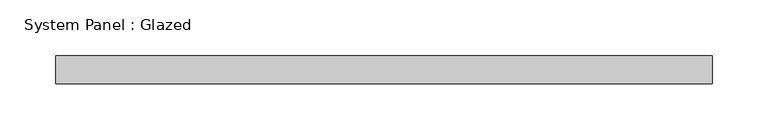
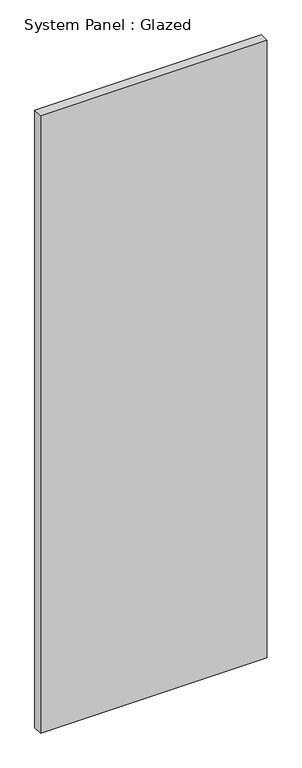
"""IFC4 building model written with IfcOpenShell, lengths in millimetres: plate geometry, System Panel : Glazed."""

from ifc_helpers import new_model, si_unit, origin, origin_with_axes, place, context, project, spatial, polyline, outline, extrude, source, transform, mapped, element, save


def system_panel_glazed_c4393626(model_context):
    return source(origin(), model_context, "Body", "SweptSolid", [
        extrude(outline(polyline([(295.6635819, 19.05), (-295.6635819, 19.05), (-295.6635819, 44.45), (295.6635819, 44.45), (295.6635819, 19.05)])), origin_with_axes(), (0.0, 0.0, 1.0), 1701.8),
    ])


if __name__ == "__main__":
    model = new_model("IFC4")
    model_context = context("Model", 3, world=origin())
    ifc_project = project(units=[si_unit("LENGTHUNIT", "METRE", prefix="MILLI")], contexts=[model_context])
    site = spatial("IfcSite", under=ifc_project)
    building = spatial("IfcBuilding", under=site)
    placement = place(None, origin())
    system_panel_glazed_shape = system_panel_glazed_c4393626(model_context)
    element("IfcPlate", 1, ObjectType="System Panel : Glazed", at=placement, inside=building, context=model_context, shape_type="MappedRepresentation", body=[
        mapped(system_panel_glazed_shape, transform((0.0, 0.0, 0.0), x_axis=(1.0, 0.0, 0.0), y_axis=(0.0, 1.0, 0.0), z_axis=(0.0, 0.0, 1.0))),
    ])
    save(model, "model.ifc")

# Revit data of these elements
# Type "System Panel : Glazed"
#   Construction Type Id = "GSP4R"
#   Analytic Construction = "1/8 in Pilkington single glazing"
#   Visual Light Transmittance = 0.9
#   Solar Heat Gain Coefficient = 0.86
#   Heat Transfer Coefficient (U) = 1.18115 BTU/(h·ft²·°F)
#   Define Thermal Properties by = 1
# Element 1 (IfcPlate, "System Panel : Glazed")
#   Materials on its faces: "Glass"
# Materials
#   "Glass": class "Glass", colour RGB 0 128 192, transparency 0.75, Description = "Soda Lime Glass", Cost = 0
